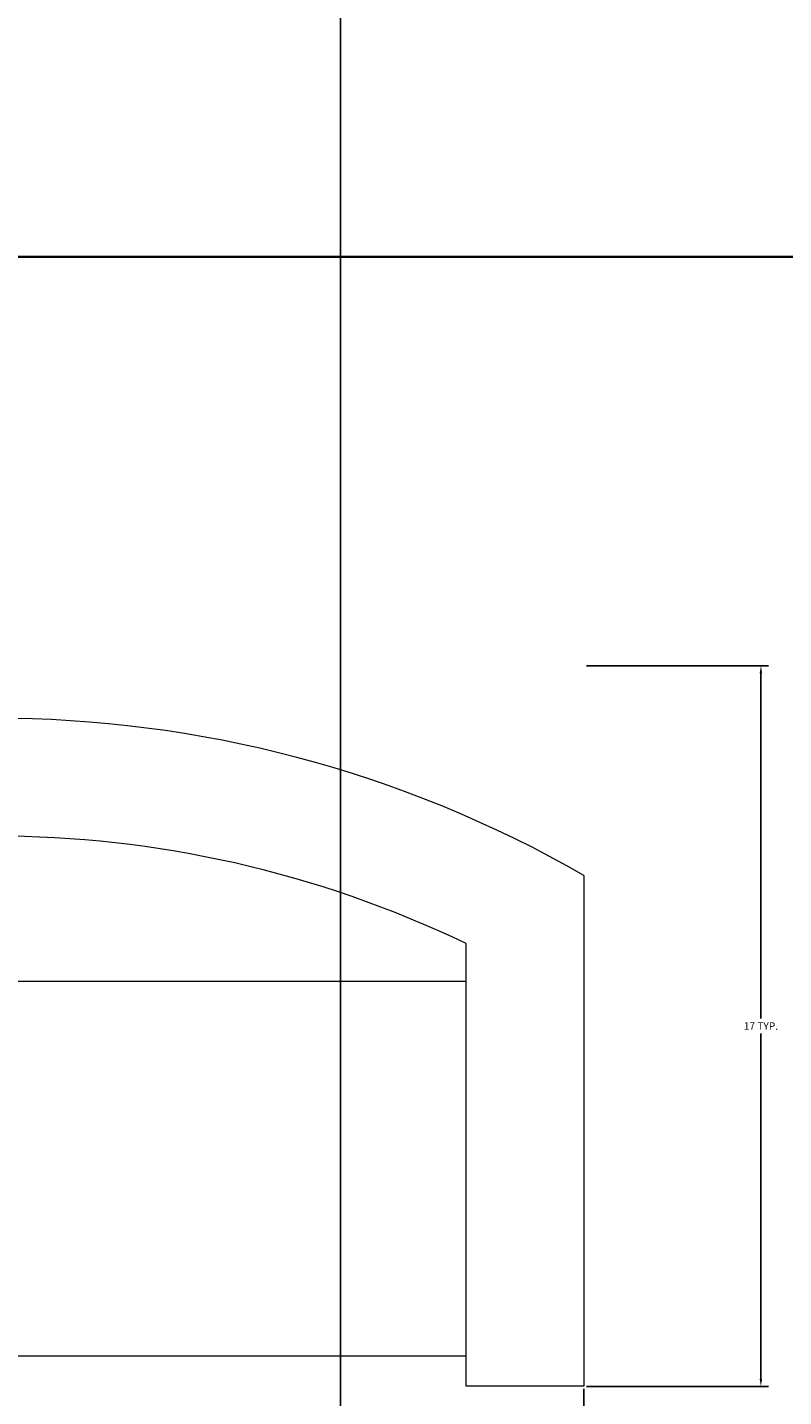
# Model space of a CAD drawing. Units: feet. Extents: x 1654 to 2985, y 1348 to 2230.
# Tile 50 of 53: x 2741 to 2759, y 1859 to 1892. Entities that reach past the tile are written whole.
import ezdxf

# ---------------------------------------------------------------- set-up
doc = ezdxf.new("R2010")
doc.units = ezdxf.units.FT
for name, color, linetype, lineweight in [('A-ANNO-DIMS', 2, 'Continuous', 18), ('A-FURN', 8, 'Continuous', 13), ('A-WALL', 7, 'Continuous', 35)]:
    doc.layers.add(name, color=color, linetype=linetype, lineweight=lineweight)
doc.styles.get("Standard").update_dxf_attribs({"font": 'arial.ttf'})
doc.dimstyles.get("Standard").update_dxf_attribs({"dimtxt": 0.18, "dimasz": 0.18, "dimexe": 0.18, "dimexo": 0.0625, "dimgap": 0.09, "dimtad": 0, "dimtih": 1, "dimtoh": 1, "dimdec": 4, "dimzin": 0, "dimdsep": 46, "dimtxsty": 'Standard', "dimcen": 0.09, "dimadec": 0, "dimazin": 0, "dimtfac": 1, "dimtdec": 4, "dimtofl": 0, "dimtmove": 0, "dimatfit": 3, "dimfxl": 1, "dimtolj": 1, "dimtzin": 0, "dimarcsym": 0})

# ---------------------------------------------------------------- blocks, each defined once
blk = doc.blocks.new('Sofa - Roundback Loveseat 5 ft.')
for p, q in [((0, -32.44198), (0, -5.99998)), ((-24, -33.99998), (-24, -11.46958)), ((24.00004, -33.99998), (24.00004, -11.46958)), ((-23.9998, -13.38178), (23.99986, -13.38178)), ((-24, -32.44198), (24.00004, -32.44198))]:
    blk.add_line(p, q)
for points in [[(-24, -33.99998), (-30, -33.99998), (-30, -7.99998)], [(30.00004, -7.99998), (30.00004, -33.99998), (24.00004, -33.99998)]]:
    blk.add_lwpolyline(points)
for centre, radius, start, end in [((0, -60.24998), 60.24998, 60.13715, 119.8628), ((0, -61.38438), 55.38444, 64.32083, 115.6792)]:
    blk.add_arc(centre, radius, start, end)
blk = doc.blocks.new('*D40')
at = {"layer": 'A-ANNO-DIMS', "color": 0, "lineweight": -2, "transparency": 16777216}
for p, q in [((2726.19, 1859.009), (2726.19, 1854.635)), ((2754.563, 1859.009), (2754.563, 1854.635)), ((2726.37, 1854.815), (2739.154, 1854.815)), ((2754.383, 1854.815), (2741.599, 1854.815))]:
    blk.add_line(p, q, dxfattribs=at)
at = {"layer": 'A-ANNO-DIMS', "color": 0, "transparency": 16777216}
for points in [[(2726.37, 1854.845), (2726.37, 1854.785), (2726.19, 1854.815)], [(2754.383, 1854.845), (2754.383, 1854.785), (2754.563, 1854.815)]]:
    blk.add_solid(points, dxfattribs=at)
at = {"layer": 'Defpoints', "color": 0, "transparency": 16777216}
for p in [(2726.19, 1859.071), (2754.563, 1859.071), (2754.563, 1854.815)]:
    blk.add_point(p, dxfattribs=at)
at = {"layer": 'A-ANNO-DIMS', "color": 0, "transparency": 16777216, "insert": (2740.376, 1854.815), "char_height": 0.18, "attachment_point": 5}
blk.add_mtext('\\A1;LOVESEAT 28 TYP.', dxfattribs=at)
blk = doc.blocks.new('*D41')
at = {"layer": 'A-ANNO-DIMS', "color": 0, "lineweight": -2, "transparency": 16777216}
for p, q in [((2754.626, 1876.411), (2758.999, 1876.411)), ((2758.819, 1876.231), (2758.819, 1867.922)), ((2758.819, 1859.251), (2758.819, 1867.561)), ((2754.626, 1859.071), (2758.999, 1859.071))]:
    blk.add_line(p, q, dxfattribs=at)
at = {"layer": 'A-ANNO-DIMS', "color": 0, "transparency": 16777216}
for points in [[(2758.789, 1876.231), (2758.849, 1876.231), (2758.819, 1876.411)], [(2758.789, 1859.251), (2758.849, 1859.251), (2758.819, 1859.071)]]:
    blk.add_solid(points, dxfattribs=at)
at = {"layer": 'Defpoints', "color": 0, "transparency": 16777216}
for p in [(2754.563, 1876.411), (2758.819, 1876.411), (2754.563, 1859.071)]:
    blk.add_point(p, dxfattribs=at)
at = {"layer": 'A-ANNO-DIMS', "color": 0, "transparency": 16777216, "insert": (2758.819, 1867.741), "char_height": 0.18, "attachment_point": 5}
blk.add_mtext('\\A1;17 TYP.', dxfattribs=at)
blk = doc.blocks.new('*D82')
at = {"layer": 'A-ANNO-DIMS', "color": 0, "lineweight": -2, "transparency": 16777216}
for p, q in [((2652.706, 2039.192), (2652.706, 1490.625)), ((2784.706, 2039.192), (2784.706, 1490.625)), ((2652.886, 1490.805), (2718.426, 1490.805)), ((2784.526, 1490.805), (2718.985, 1490.805))]:
    blk.add_line(p, q, dxfattribs=at)
at = {"layer": 'A-ANNO-DIMS', "color": 0, "transparency": 16777216}
for points in [[(2652.886, 1490.835), (2652.886, 1490.775), (2652.706, 1490.805)], [(2784.526, 1490.835), (2784.526, 1490.775), (2784.706, 1490.805)]]:
    blk.add_solid(points, dxfattribs=at)
at = {"layer": 'Defpoints', "color": 0, "transparency": 16777216}
for p in [(2652.706, 2039.255), (2784.706, 2039.255), (2784.706, 1490.805)]:
    blk.add_point(p, dxfattribs=at)
at = {"layer": 'A-ANNO-DIMS', "color": 0, "transparency": 16777216, "insert": (2718.706, 1490.805), "char_height": 0.18, "attachment_point": 5}
blk.add_mtext('\\A1;132', dxfattribs=at)
blk = doc.blocks.new('*D86')
at = {"layer": 'A-ANNO-DIMS', "color": 0, "lineweight": -2, "transparency": 16777216}
for p, q in [((2748.706, 1616.317), (2748.706, 2149.885)), ((2784.706, 1607.317), (2784.706, 2149.885)), ((2748.886, 2149.705), (2766.487, 2149.705)), ((2784.526, 2149.705), (2766.925, 2149.705))]:
    blk.add_line(p, q, dxfattribs=at)
at = {"layer": 'A-ANNO-DIMS', "color": 0, "transparency": 16777216}
for points in [[(2748.886, 2149.735), (2748.886, 2149.675), (2748.706, 2149.705)], [(2784.526, 2149.735), (2784.526, 2149.675), (2784.706, 2149.705)]]:
    blk.add_solid(points, dxfattribs=at)
at = {"layer": 'Defpoints', "color": 0, "transparency": 16777216}
for p in [(2784.706, 2149.705), (2748.706, 1616.255), (2784.706, 1607.255)]:
    blk.add_point(p, dxfattribs=at)
at = {"layer": 'A-ANNO-DIMS', "color": 0, "transparency": 16777216, "insert": (2766.706, 2149.705), "char_height": 0.18, "attachment_point": 5}
blk.add_mtext('\\A1;36', dxfattribs=at)

msp = doc.modelspace()

# ---------------------------------------------------------------- linework, layer by layer
at = {"layer": 'A-WALL'}
msp.add_line((2784.7058, 1886.2549), (2652.7058, 1886.2549), dxfattribs=at)

# ---------------------------------------------------------------- block references
at = {"layer": 'A-FURN', "xscale": 0.4728872769476647, "yscale": 0.4728872769476647, "zscale": 0.4728872769476647}
msp.add_blockref('Sofa - Roundback Loveseat 5 ft.', (2740.3765, 1875.1496), dxfattribs=at)

# ---------------------------------------------------------------- dimensions: what is measured, and where the dimension line sits
at = {"layer": 'A-ANNO-DIMS'}
for base, p1, p2, picture, middle in [((2784.7058, 2149.7049), (2748.7058, 1616.2549), (2784.7058, 1607.2549), '*D86', (2766.7058, 2149.7049)), ((2784.7058, 1490.8049), (2652.7058, 2039.2549), (2784.7058, 2039.2549), '*D82', (2718.7058, 1490.8049))]:
    dim = msp.add_linear_dim(base=base, p1=p1, p2=p2, dimstyle='Standard', override={"dimdec": 0, "dimlfac": 1, "dimrnd": 0, "dimzin": 0, "dimdsep": 46, "dimlunit": 2}, dxfattribs=at)
    dim.commit()
    dim.dimension.update_dxf_attribs({"geometry": picture, "text_midpoint": middle})
dim = msp.add_linear_dim(base=(2758.8191, 1876.4107), p1=(2754.5631, 1859.0715), p2=(2754.5631, 1876.4107), angle=90, text='<> TYP.', dimstyle='Standard', override={"dimdec": 0, "dimlfac": 1, "dimrnd": 0, "dimzin": 0, "dimdsep": 46, "dimlunit": 2}, dxfattribs=at)
dim.commit()
dim.dimension.update_dxf_attribs({"geometry": '*D41', "text_midpoint": (2758.8191, 1867.7411)})
dim = msp.add_linear_dim(base=(2754.5631, 1854.8155), p1=(2726.1899, 1859.0715), p2=(2754.5631, 1859.0715), text='LOVESEAT <> TYP.', dimstyle='Standard', override={"dimdec": 0, "dimlfac": 1, "dimrnd": 0, "dimzin": 0, "dimdsep": 46, "dimlunit": 2}, dxfattribs=at)
dim.commit()
dim.dimension.update_dxf_attribs({"geometry": '*D40', "text_midpoint": (2740.3765, 1854.8155)})

doc.saveas('drawing.dxf')
